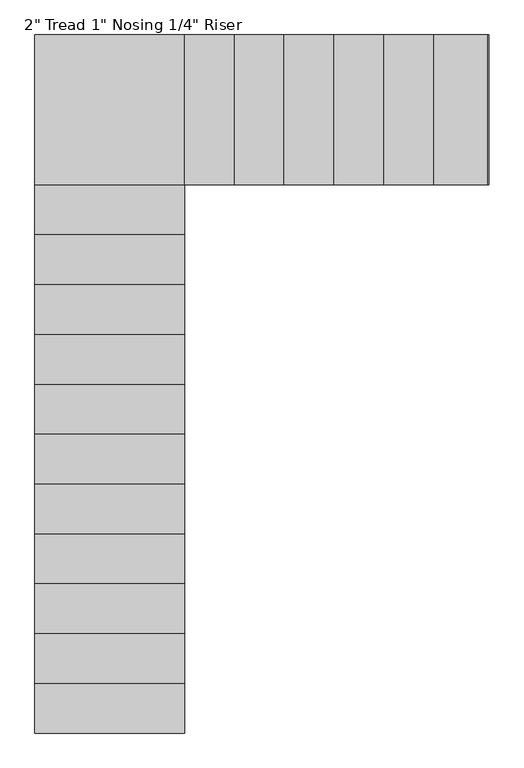
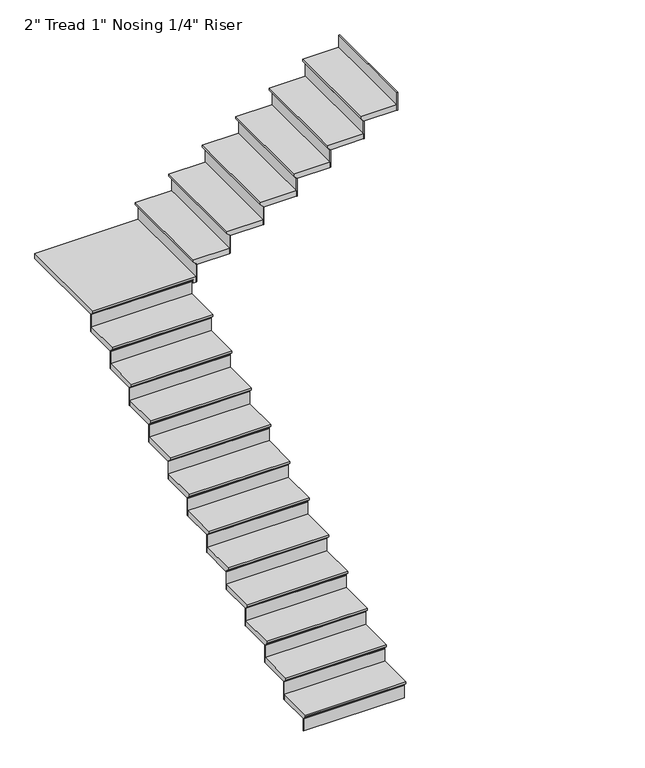
"""IFC4 building model written with IfcOpenShell, lengths in millimetres: stair flight geometry."""

from ifc_helpers import new_model, si_unit, origin, place, context, project, spatial, faceted_brep, source, transform, mapped, element, save


def stair_flight_5b7f780d(model_context):
    return source(origin(), model_context, "Body", "Brep", [
        faceted_brep([(-8401.1607439, -642.5827462, 455.0833333), (-8401.1607439, -642.5827462, 474.1333333), (-9317.1482439, -642.5827462, 474.1333333), (-9317.1482439, -642.5827462, 455.0833333), (-8401.1607439, -617.1827462, 429.6833333), (-9317.1482439, -617.1827462, 429.6833333), (-8401.1607439, -312.3827462, 474.1333333), (-9317.1482439, -312.3827462, 474.1333333), (-9317.1482439, -617.1827462, 423.3333333), (-9317.1482439, -312.3827462, 423.3333333), (-8401.1607439, -312.3827462, 423.3333333), (-8401.1607439, -617.1827462, 423.3333333)], [[[0, 1, 2, 3]], [[4, 0, 3, 5]], [[2, 1, 6, 7]], [[8, 9, 10, 11]], [[2, 7, 9, 8, 5, 3]], [[8, 11, 4, 5]], [[6, 1, 0, 4, 11, 10]], [[7, 6, 10, 9]]]),
        faceted_brep([(-8401.1607439, -617.1827462, 423.3333333), (-8401.1607439, -617.1827462, 304.8), (-8401.1607439, -610.8327462, 304.8), (-8401.1607439, -610.8327462, 423.3333333), (-9317.1482439, -617.1827462, 423.3333333), (-9317.1482439, -610.8327462, 423.3333333), (-9317.1482439, -610.8327462, 304.8), (-9317.1482439, -617.1827462, 304.8)], [[[0, 1, 2, 3]], [[4, 5, 6, 7]], [[1, 0, 4, 7]], [[2, 1, 7, 6]], [[3, 2, 6, 5]], [[0, 3, 5, 4]]]),
        faceted_brep([(-8401.1607439, -312.3827462, 592.6666667), (-8401.1607439, -312.3827462, 423.3333333), (-8401.1607439, -306.0327462, 423.3333333), (-8401.1607439, -306.0327462, 592.6666667), (-9317.1482439, -312.3827462, 592.6666667), (-9317.1482439, -306.0327462, 592.6666667), (-9317.1482439, -306.0327462, 423.3333333), (-9317.1482439, -312.3827462, 423.3333333)], [[[0, 1, 2, 3]], [[4, 5, 6, 7]], [[1, 0, 4, 7]], [[2, 1, 7, 6]], [[3, 2, 6, 5]], [[0, 3, 5, 4]]]),
        faceted_brep([(-9317.1482439, -337.7827462, 643.4666667), (-8401.1607439, -337.7827462, 643.4666667), (-8401.1607439, -7.5827462, 643.4666667), (-9317.1482439, -7.5827462, 643.4666667), (-9317.1482439, -312.3827462, 592.6666667), (-9317.1482439, -7.5827462, 592.6666667), (-8401.1607439, -7.5827462, 592.6666667), (-8401.1607439, -312.3827462, 592.6666667), (-9317.1482439, -312.3827462, 599.0166667), (-9317.1482439, -337.7827462, 624.4166667), (-8401.1607439, -312.3827462, 599.0166667), (-8401.1607439, -337.7827462, 624.4166667)], [[[0, 1, 2, 3]], [[4, 5, 6, 7]], [[0, 3, 5, 4, 8, 9]], [[4, 7, 10, 8]], [[2, 1, 11, 10, 7, 6]], [[3, 2, 6, 5]], [[11, 1, 0, 9]], [[10, 11, 9, 8]]]),
        faceted_brep([(-8401.1607439, -7.5827462, 762.0), (-8401.1607439, -7.5827462, 592.6666667), (-8401.1607439, -1.2327462, 592.6666667), (-8401.1607439, -1.2327462, 762.0), (-9317.1482439, -7.5827462, 762.0), (-9317.1482439, -1.2327462, 762.0), (-9317.1482439, -1.2327462, 592.6666667), (-9317.1482439, -7.5827462, 592.6666667)], [[[0, 1, 2, 3]], [[4, 5, 6, 7]], [[1, 0, 4, 7]], [[2, 1, 7, 6]], [[3, 2, 6, 5]], [[0, 3, 5, 4]]]),
        faceted_brep([(-9317.1482439, -32.9827462, 812.8), (-8401.1607439, -32.9827462, 812.8), (-8401.1607439, 297.2172538, 812.8), (-9317.1482439, 297.2172538, 812.8), (-9317.1482439, -7.5827462, 762.0), (-9317.1482439, 297.2172538, 762.0), (-8401.1607439, 297.2172538, 762.0), (-8401.1607439, -7.5827462, 762.0), (-9317.1482439, -7.5827462, 768.35), (-9317.1482439, -32.9827462, 793.75), (-8401.1607439, -7.5827462, 768.35), (-8401.1607439, -32.9827462, 793.75)], [[[0, 1, 2, 3]], [[4, 5, 6, 7]], [[0, 3, 5, 4, 8, 9]], [[4, 7, 10, 8]], [[2, 1, 11, 10, 7, 6]], [[3, 2, 6, 5]], [[11, 1, 0, 9]], [[10, 11, 9, 8]]]),
        faceted_brep([(-8401.1607439, 297.2172538, 931.3333333), (-8401.1607439, 297.2172538, 762.0), (-8401.1607439, 303.5672538, 762.0), (-8401.1607439, 303.5672538, 931.3333333), (-9317.1482439, 297.2172538, 931.3333333), (-9317.1482439, 303.5672538, 931.3333333), (-9317.1482439, 303.5672538, 762.0), (-9317.1482439, 297.2172538, 762.0)], [[[0, 1, 2, 3]], [[4, 5, 6, 7]], [[1, 0, 4, 7]], [[2, 1, 7, 6]], [[3, 2, 6, 5]], [[0, 3, 5, 4]]]),
        faceted_brep([(-9317.1482439, 271.8172538, 982.1333333), (-8401.1607439, 271.8172538, 982.1333333), (-8401.1607439, 602.0172538, 982.1333333), (-9317.1482439, 602.0172538, 982.1333333), (-9317.1482439, 297.2172538, 931.3333333), (-9317.1482439, 602.0172538, 931.3333333), (-8401.1607439, 602.0172538, 931.3333333), (-8401.1607439, 297.2172538, 931.3333333), (-9317.1482439, 297.2172538, 937.6833333), (-9317.1482439, 271.8172538, 963.0833333), (-8401.1607439, 297.2172538, 937.6833333), (-8401.1607439, 271.8172538, 963.0833333)], [[[0, 1, 2, 3]], [[4, 5, 6, 7]], [[0, 3, 5, 4, 8, 9]], [[4, 7, 10, 8]], [[2, 1, 11, 10, 7, 6]], [[3, 2, 6, 5]], [[11, 1, 0, 9]], [[10, 11, 9, 8]]]),
        faceted_brep([(-8401.1607439, 602.0172538, 1100.6666667), (-8401.1607439, 602.0172538, 931.3333333), (-8401.1607439, 608.3672538, 931.3333333), (-8401.1607439, 608.3672538, 1100.6666667), (-9317.1482439, 602.0172538, 1100.6666667), (-9317.1482439, 608.3672538, 1100.6666667), (-9317.1482439, 608.3672538, 931.3333333), (-9317.1482439, 602.0172538, 931.3333333)], [[[0, 1, 2, 3]], [[4, 5, 6, 7]], [[1, 0, 4, 7]], [[2, 1, 7, 6]], [[3, 2, 6, 5]], [[0, 3, 5, 4]]]),
        faceted_brep([(-9317.1482439, 576.6172538, 1151.4666667), (-8401.1607439, 576.6172538, 1151.4666667), (-8401.1607439, 906.8172538, 1151.4666667), (-9317.1482439, 906.8172538, 1151.4666667), (-9317.1482439, 602.0172538, 1100.6666667), (-9317.1482439, 906.8172538, 1100.6666667), (-8401.1607439, 906.8172538, 1100.6666667), (-8401.1607439, 602.0172538, 1100.6666667), (-9317.1482439, 602.0172538, 1107.0166667), (-9317.1482439, 576.6172538, 1132.4166667), (-8401.1607439, 602.0172538, 1107.0166667), (-8401.1607439, 576.6172538, 1132.4166667)], [[[0, 1, 2, 3]], [[4, 5, 6, 7]], [[0, 3, 5, 4, 8, 9]], [[4, 7, 10, 8]], [[2, 1, 11, 10, 7, 6]], [[3, 2, 6, 5]], [[11, 1, 0, 9]], [[10, 11, 9, 8]]]),
        faceted_brep([(-8401.1607439, 906.8172538, 1270.0), (-8401.1607439, 906.8172538, 1100.6666667), (-8401.1607439, 913.1672538, 1100.6666667), (-8401.1607439, 913.1672538, 1270.0), (-9317.1482439, 906.8172538, 1270.0), (-9317.1482439, 913.1672538, 1270.0), (-9317.1482439, 913.1672538, 1100.6666667), (-9317.1482439, 906.8172538, 1100.6666667)], [[[0, 1, 2, 3]], [[4, 5, 6, 7]], [[1, 0, 4, 7]], [[2, 1, 7, 6]], [[3, 2, 6, 5]], [[0, 3, 5, 4]]]),
        faceted_brep([(-9317.1482439, 881.4172538, 1320.8), (-8401.1607439, 881.4172538, 1320.8), (-8401.1607439, 1211.6172538, 1320.8), (-9317.1482439, 1211.6172538, 1320.8), (-9317.1482439, 906.8172538, 1270.0), (-9317.1482439, 1211.6172538, 1270.0), (-8401.1607439, 1211.6172538, 1270.0), (-8401.1607439, 906.8172538, 1270.0), (-9317.1482439, 906.8172538, 1276.35), (-9317.1482439, 881.4172538, 1301.75), (-8401.1607439, 906.8172538, 1276.35), (-8401.1607439, 881.4172538, 1301.75)], [[[0, 1, 2, 3]], [[4, 5, 6, 7]], [[0, 3, 5, 4, 8, 9]], [[4, 7, 10, 8]], [[2, 1, 11, 10, 7, 6]], [[3, 2, 6, 5]], [[11, 1, 0, 9]], [[10, 11, 9, 8]]]),
        faceted_brep([(-8401.1607439, 1211.6172538, 1439.3333333), (-8401.1607439, 1211.6172538, 1270.0), (-8401.1607439, 1217.9672538, 1270.0), (-8401.1607439, 1217.9672538, 1439.3333333), (-9317.1482439, 1211.6172538, 1439.3333333), (-9317.1482439, 1217.9672538, 1439.3333333), (-9317.1482439, 1217.9672538, 1270.0), (-9317.1482439, 1211.6172538, 1270.0)], [[[0, 1, 2, 3]], [[4, 5, 6, 7]], [[1, 0, 4, 7]], [[2, 1, 7, 6]], [[3, 2, 6, 5]], [[0, 3, 5, 4]]]),
        faceted_brep([(-9317.1482439, 1186.2172538, 1490.1333333), (-8401.1607439, 1186.2172538, 1490.1333333), (-8401.1607439, 1516.4172538, 1490.1333333), (-9317.1482439, 1516.4172538, 1490.1333333), (-9317.1482439, 1211.6172538, 1439.3333333), (-9317.1482439, 1516.4172538, 1439.3333333), (-8401.1607439, 1516.4172538, 1439.3333333), (-8401.1607439, 1211.6172538, 1439.3333333), (-9317.1482439, 1211.6172538, 1445.6833333), (-9317.1482439, 1186.2172538, 1471.0833333), (-8401.1607439, 1211.6172538, 1445.6833333), (-8401.1607439, 1186.2172538, 1471.0833333)], [[[0, 1, 2, 3]], [[4, 5, 6, 7]], [[0, 3, 5, 4, 8, 9]], [[4, 7, 10, 8]], [[2, 1, 11, 10, 7, 6]], [[3, 2, 6, 5]], [[11, 1, 0, 9]], [[10, 11, 9, 8]]]),
        faceted_brep([(-8401.1607439, 1516.4172538, 1608.6666667), (-8401.1607439, 1516.4172538, 1439.3333333), (-8401.1607439, 1522.7672538, 1439.3333333), (-8401.1607439, 1522.7672538, 1608.6666667), (-9317.1482439, 1516.4172538, 1608.6666667), (-9317.1482439, 1522.7672538, 1608.6666667), (-9317.1482439, 1522.7672538, 1439.3333333), (-9317.1482439, 1516.4172538, 1439.3333333)], [[[0, 1, 2, 3]], [[4, 5, 6, 7]], [[1, 0, 4, 7]], [[2, 1, 7, 6]], [[3, 2, 6, 5]], [[0, 3, 5, 4]]]),
        faceted_brep([(-9317.1482439, 1491.0172538, 1659.4666667), (-8401.1607439, 1491.0172538, 1659.4666667), (-8401.1607439, 1821.2172538, 1659.4666667), (-9317.1482439, 1821.2172538, 1659.4666667), (-9317.1482439, 1516.4172538, 1608.6666667), (-9317.1482439, 1821.2172538, 1608.6666667), (-8401.1607439, 1821.2172538, 1608.6666667), (-8401.1607439, 1516.4172538, 1608.6666667), (-9317.1482439, 1516.4172538, 1615.0166667), (-9317.1482439, 1491.0172538, 1640.4166667), (-8401.1607439, 1516.4172538, 1615.0166667), (-8401.1607439, 1491.0172538, 1640.4166667)], [[[0, 1, 2, 3]], [[4, 5, 6, 7]], [[0, 3, 5, 4, 8, 9]], [[4, 7, 10, 8]], [[2, 1, 11, 10, 7, 6]], [[3, 2, 6, 5]], [[11, 1, 0, 9]], [[10, 11, 9, 8]]]),
        faceted_brep([(-8401.1607439, 1821.2172538, 1778.0), (-8401.1607439, 1821.2172538, 1608.6666667), (-8401.1607439, 1827.5672538, 1608.6666667), (-8401.1607439, 1827.5672538, 1778.0), (-9317.1482439, 1821.2172538, 1778.0), (-9317.1482439, 1827.5672538, 1778.0), (-9317.1482439, 1827.5672538, 1608.6666667), (-9317.1482439, 1821.2172538, 1608.6666667)], [[[0, 1, 2, 3]], [[4, 5, 6, 7]], [[1, 0, 4, 7]], [[2, 1, 7, 6]], [[3, 2, 6, 5]], [[0, 3, 5, 4]]]),
        faceted_brep([(-9317.1482439, 1795.8172538, 1828.8), (-8401.1607439, 1795.8172538, 1828.8), (-8401.1607439, 2126.0172538, 1828.8), (-9317.1482439, 2126.0172538, 1828.8), (-9317.1482439, 1821.2172538, 1778.0), (-9317.1482439, 2126.0172538, 1778.0), (-8401.1607439, 2126.0172538, 1778.0), (-8401.1607439, 1821.2172538, 1778.0), (-9317.1482439, 1821.2172538, 1784.35), (-9317.1482439, 1795.8172538, 1809.75), (-8401.1607439, 1821.2172538, 1784.35), (-8401.1607439, 1795.8172538, 1809.75)], [[[0, 1, 2, 3]], [[4, 5, 6, 7]], [[0, 3, 5, 4, 8, 9]], [[4, 7, 10, 8]], [[2, 1, 11, 10, 7, 6]], [[3, 2, 6, 5]], [[11, 1, 0, 9]], [[10, 11, 9, 8]]]),
        faceted_brep([(-8401.1607439, 2126.0172538, 1947.3333333), (-8401.1607439, 2126.0172538, 1778.0), (-8401.1607439, 2132.3672538, 1778.0), (-8401.1607439, 2132.3672538, 1947.3333333), (-9317.1482439, 2126.0172538, 1947.3333333), (-9317.1482439, 2132.3672538, 1947.3333333), (-9317.1482439, 2132.3672538, 1778.0), (-9317.1482439, 2126.0172538, 1778.0)], [[[0, 1, 2, 3]], [[4, 5, 6, 7]], [[1, 0, 4, 7]], [[2, 1, 7, 6]], [[3, 2, 6, 5]], [[0, 3, 5, 4]]]),
        faceted_brep([(-9317.1482439, 2100.6172538, 1998.1333333), (-8401.1607439, 2100.6172538, 1998.1333333), (-8401.1607439, 2430.8172538, 1998.1333333), (-9317.1482439, 2430.8172538, 1998.1333333), (-9317.1482439, 2126.0172538, 1947.3333333), (-9317.1482439, 2430.8172538, 1947.3333333), (-8401.1607439, 2430.8172538, 1947.3333333), (-8401.1607439, 2126.0172538, 1947.3333333), (-9317.1482439, 2126.0172538, 1953.6833333), (-9317.1482439, 2100.6172538, 1979.0833333), (-8401.1607439, 2126.0172538, 1953.6833333), (-8401.1607439, 2100.6172538, 1979.0833333)], [[[0, 1, 2, 3]], [[4, 5, 6, 7]], [[0, 3, 5, 4, 8, 9]], [[4, 7, 10, 8]], [[2, 1, 11, 10, 7, 6]], [[3, 2, 6, 5]], [[11, 1, 0, 9]], [[10, 11, 9, 8]]]),
        faceted_brep([(-8401.1607439, 2430.8172538, 2116.6666667), (-8401.1607439, 2430.8172538, 1947.3333333), (-8401.1607439, 2437.1672538, 1947.3333333), (-8401.1607439, 2437.1672538, 2116.6666667), (-9317.1482439, 2430.8172538, 2116.6666667), (-9317.1482439, 2437.1672538, 2116.6666667), (-9317.1482439, 2437.1672538, 1947.3333333), (-9317.1482439, 2430.8172538, 1947.3333333)], [[[0, 1, 2, 3]], [[4, 5, 6, 7]], [[1, 0, 4, 7]], [[2, 1, 7, 6]], [[3, 2, 6, 5]], [[0, 3, 5, 4]]]),
        faceted_brep([(-9317.1482439, 2405.4172538, 2167.4666667), (-8401.1607439, 2405.4172538, 2167.4666667), (-8401.1607439, 2735.6172538, 2167.4666667), (-9317.1482439, 2735.6172538, 2167.4666667), (-9317.1482439, 2430.8172538, 2116.6666667), (-9317.1482439, 2735.6172538, 2116.6666667), (-8401.1607439, 2735.6172538, 2116.6666667), (-8401.1607439, 2430.8172538, 2116.6666667), (-9317.1482439, 2430.8172538, 2123.0166667), (-9317.1482439, 2405.4172538, 2148.4166667), (-8401.1607439, 2430.8172538, 2123.0166667), (-8401.1607439, 2405.4172538, 2148.4166667)], [[[0, 1, 2, 3]], [[4, 5, 6, 7]], [[0, 3, 5, 4, 8, 9]], [[4, 7, 10, 8]], [[2, 1, 11, 10, 7, 6]], [[3, 2, 6, 5]], [[11, 1, 0, 9]], [[10, 11, 9, 8]]]),
        faceted_brep([(-8401.1607439, 2735.6172538, 2286.0), (-8401.1607439, 2735.6172538, 2116.6666667), (-8401.1607439, 2741.9672538, 2116.6666667), (-8401.1607439, 2741.9672538, 2286.0), (-9317.1482439, 2735.6172538, 2286.0), (-9317.1482439, 2741.9672538, 2286.0), (-9317.1482439, 2741.9672538, 2116.6666667), (-9317.1482439, 2735.6172538, 2116.6666667)], [[[0, 1, 2, 3]], [[4, 5, 6, 7]], [[1, 0, 4, 7]], [[2, 1, 7, 6]], [[3, 2, 6, 5]], [[0, 3, 5, 4]]]),
        faceted_brep([(-8375.7607439, 3624.6172538, 2336.8), (-9317.1482439, 3624.6172538, 2336.8), (-9317.1482439, 2710.2172538, 2336.8), (-8375.7607439, 2710.2172538, 2336.8), (-9317.1482439, 3624.6172538, 2286.0), (-8375.7607439, 3624.6172538, 2286.0), (-8375.7607439, 2710.2172538, 2286.0), (-8401.1607439, 2710.2172538, 2286.0), (-8401.1607439, 2735.6172538, 2286.0), (-9317.1482439, 2735.6172538, 2286.0), (-9317.1482439, 2735.6172538, 2292.35), (-9317.1482439, 2710.2172538, 2317.75), (-8401.1607439, 2735.6172538, 2292.35), (-8401.1607439, 2710.2172538, 2317.75)], [[[0, 1, 2, 3]], [[4, 5, 6, 7, 8, 9]], [[1, 0, 5, 4]], [[2, 1, 4, 9, 10, 11]], [[9, 8, 12, 10]], [[8, 7, 13, 12]], [[3, 2, 11, 13, 7, 6]], [[0, 3, 6, 5]], [[11, 10, 12, 13]]]),
        faceted_brep([(-8375.7607439, 2710.2172538, 2455.3333333), (-8375.7607439, 2710.2172538, 2286.0), (-8369.4107439, 2710.2172538, 2286.0), (-8369.4107439, 2710.2172538, 2455.3333333), (-8375.7607439, 3624.6172538, 2455.3333333), (-8369.4107439, 3624.6172538, 2455.3333333), (-8369.4107439, 3624.6172538, 2286.0), (-8375.7607439, 3624.6172538, 2286.0)], [[[0, 1, 2, 3]], [[4, 5, 6, 7]], [[1, 0, 4, 7]], [[2, 1, 7, 6]], [[3, 2, 6, 5]], [[0, 3, 5, 4]]]),
        faceted_brep([(-8401.1607439, 3624.6172538, 2506.1333333), (-8401.1607439, 2710.2172538, 2506.1333333), (-8070.9607439, 2710.2172538, 2506.1333333), (-8070.9607439, 3624.6172538, 2506.1333333), (-8375.7607439, 3624.6172538, 2455.3333333), (-8070.9607439, 3624.6172538, 2455.3333333), (-8070.9607439, 2710.2172538, 2455.3333333), (-8375.7607439, 2710.2172538, 2455.3333333), (-8375.7607439, 3624.6172538, 2461.6833333), (-8401.1607439, 3624.6172538, 2487.0833333), (-8375.7607439, 2710.2172538, 2461.6833333), (-8401.1607439, 2710.2172538, 2487.0833333)], [[[0, 1, 2, 3]], [[4, 5, 6, 7]], [[0, 3, 5, 4, 8, 9]], [[4, 7, 10, 8]], [[2, 1, 11, 10, 7, 6]], [[3, 2, 6, 5]], [[11, 1, 0, 9]], [[10, 11, 9, 8]]]),
        faceted_brep([(-8070.9607439, 2710.2172538, 2624.6666667), (-8070.9607439, 2710.2172538, 2455.3333333), (-8064.6107439, 2710.2172538, 2455.3333333), (-8064.6107439, 2710.2172538, 2624.6666667), (-8070.9607439, 3624.6172538, 2624.6666667), (-8064.6107439, 3624.6172538, 2624.6666667), (-8064.6107439, 3624.6172538, 2455.3333333), (-8070.9607439, 3624.6172538, 2455.3333333)], [[[0, 1, 2, 3]], [[4, 5, 6, 7]], [[1, 0, 4, 7]], [[2, 1, 7, 6]], [[3, 2, 6, 5]], [[0, 3, 5, 4]]]),
        faceted_brep([(-8096.3607439, 3624.6172538, 2675.4666667), (-8096.3607439, 2710.2172538, 2675.4666667), (-7766.1607439, 2710.2172538, 2675.4666667), (-7766.1607439, 3624.6172538, 2675.4666667), (-8070.9607439, 3624.6172538, 2624.6666667), (-7766.1607439, 3624.6172538, 2624.6666667), (-7766.1607439, 2710.2172538, 2624.6666667), (-8070.9607439, 2710.2172538, 2624.6666667), (-8070.9607439, 3624.6172538, 2631.0166667), (-8096.3607439, 3624.6172538, 2656.4166667), (-8070.9607439, 2710.2172538, 2631.0166667), (-8096.3607439, 2710.2172538, 2656.4166667)], [[[0, 1, 2, 3]], [[4, 5, 6, 7]], [[0, 3, 5, 4, 8, 9]], [[4, 7, 10, 8]], [[2, 1, 11, 10, 7, 6]], [[3, 2, 6, 5]], [[11, 1, 0, 9]], [[10, 11, 9, 8]]]),
        faceted_brep([(-7766.1607439, 2710.2172538, 2794.0), (-7766.1607439, 2710.2172538, 2624.6666667), (-7759.8107439, 2710.2172538, 2624.6666667), (-7759.8107439, 2710.2172538, 2794.0), (-7766.1607439, 3624.6172538, 2794.0), (-7759.8107439, 3624.6172538, 2794.0), (-7759.8107439, 3624.6172538, 2624.6666667), (-7766.1607439, 3624.6172538, 2624.6666667)], [[[0, 1, 2, 3]], [[4, 5, 6, 7]], [[1, 0, 4, 7]], [[2, 1, 7, 6]], [[3, 2, 6, 5]], [[0, 3, 5, 4]]]),
        faceted_brep([(-7791.5607439, 3624.6172538, 2844.8), (-7791.5607439, 2710.2172538, 2844.8), (-7461.3607439, 2710.2172538, 2844.8), (-7461.3607439, 3624.6172538, 2844.8), (-7766.1607439, 3624.6172538, 2794.0), (-7461.3607439, 3624.6172538, 2794.0), (-7461.3607439, 2710.2172538, 2794.0), (-7766.1607439, 2710.2172538, 2794.0), (-7766.1607439, 3624.6172538, 2800.35), (-7791.5607439, 3624.6172538, 2825.75), (-7766.1607439, 2710.2172538, 2800.35), (-7791.5607439, 2710.2172538, 2825.75)], [[[0, 1, 2, 3]], [[4, 5, 6, 7]], [[0, 3, 5, 4, 8, 9]], [[4, 7, 10, 8]], [[2, 1, 11, 10, 7, 6]], [[3, 2, 6, 5]], [[11, 1, 0, 9]], [[10, 11, 9, 8]]]),
        faceted_brep([(-7461.3607439, 2710.2172538, 2963.3333333), (-7461.3607439, 2710.2172538, 2794.0), (-7455.0107439, 2710.2172538, 2794.0), (-7455.0107439, 2710.2172538, 2963.3333333), (-7461.3607439, 3624.6172538, 2963.3333333), (-7455.0107439, 3624.6172538, 2963.3333333), (-7455.0107439, 3624.6172538, 2794.0), (-7461.3607439, 3624.6172538, 2794.0)], [[[0, 1, 2, 3]], [[4, 5, 6, 7]], [[1, 0, 4, 7]], [[2, 1, 7, 6]], [[3, 2, 6, 5]], [[0, 3, 5, 4]]]),
        faceted_brep([(-7486.7607439, 3624.6172538, 3014.1333333), (-7486.7607439, 2710.2172538, 3014.1333333), (-7156.5607439, 2710.2172538, 3014.1333333), (-7156.5607439, 3624.6172538, 3014.1333333), (-7461.3607439, 3624.6172538, 2963.3333333), (-7156.5607439, 3624.6172538, 2963.3333333), (-7156.5607439, 2710.2172538, 2963.3333333), (-7461.3607439, 2710.2172538, 2963.3333333), (-7461.3607439, 3624.6172538, 2969.6833333), (-7486.7607439, 3624.6172538, 2995.0833333), (-7461.3607439, 2710.2172538, 2969.6833333), (-7486.7607439, 2710.2172538, 2995.0833333)], [[[0, 1, 2, 3]], [[4, 5, 6, 7]], [[0, 3, 5, 4, 8, 9]], [[4, 7, 10, 8]], [[2, 1, 11, 10, 7, 6]], [[3, 2, 6, 5]], [[11, 1, 0, 9]], [[10, 11, 9, 8]]]),
        faceted_brep([(-7156.5607439, 2710.2172538, 3132.6666667), (-7156.5607439, 2710.2172538, 2963.3333333), (-7150.2107439, 2710.2172538, 2963.3333333), (-7150.2107439, 2710.2172538, 3132.6666667), (-7156.5607439, 3624.6172538, 3132.6666667), (-7150.2107439, 3624.6172538, 3132.6666667), (-7150.2107439, 3624.6172538, 2963.3333333), (-7156.5607439, 3624.6172538, 2963.3333333)], [[[0, 1, 2, 3]], [[4, 5, 6, 7]], [[1, 0, 4, 7]], [[2, 1, 7, 6]], [[3, 2, 6, 5]], [[0, 3, 5, 4]]]),
        faceted_brep([(-7181.9607439, 3624.6172538, 3183.4666667), (-7181.9607439, 2710.2172538, 3183.4666667), (-6851.7607439, 2710.2172538, 3183.4666667), (-6851.7607439, 3624.6172538, 3183.4666667), (-7156.5607439, 3624.6172538, 3132.6666667), (-6851.7607439, 3624.6172538, 3132.6666667), (-6851.7607439, 2710.2172538, 3132.6666667), (-7156.5607439, 2710.2172538, 3132.6666667), (-7156.5607439, 3624.6172538, 3139.0166667), (-7181.9607439, 3624.6172538, 3164.4166667), (-7156.5607439, 2710.2172538, 3139.0166667), (-7181.9607439, 2710.2172538, 3164.4166667)], [[[0, 1, 2, 3]], [[4, 5, 6, 7]], [[0, 3, 5, 4, 8, 9]], [[4, 7, 10, 8]], [[2, 1, 11, 10, 7, 6]], [[3, 2, 6, 5]], [[11, 1, 0, 9]], [[10, 11, 9, 8]]]),
        faceted_brep([(-6851.7607439, 2710.2172538, 3302.0), (-6851.7607439, 2710.2172538, 3132.6666667), (-6845.4107439, 2710.2172538, 3132.6666667), (-6845.4107439, 2710.2172538, 3302.0), (-6851.7607439, 3624.6172538, 3302.0), (-6845.4107439, 3624.6172538, 3302.0), (-6845.4107439, 3624.6172538, 3132.6666667), (-6851.7607439, 3624.6172538, 3132.6666667)], [[[0, 1, 2, 3]], [[4, 5, 6, 7]], [[1, 0, 4, 7]], [[2, 1, 7, 6]], [[3, 2, 6, 5]], [[0, 3, 5, 4]]]),
        faceted_brep([(-6546.9607439, 2710.2172538, 3471.3333333), (-6546.9607439, 2710.2172538, 3302.0), (-6540.6107439, 2710.2172538, 3302.0), (-6540.6107439, 2710.2172538, 3471.3333333), (-6546.9607439, 3624.6172538, 3471.3333333), (-6540.6107439, 3624.6172538, 3471.3333333), (-6540.6107439, 3624.6172538, 3302.0), (-6546.9607439, 3624.6172538, 3302.0)], [[[0, 1, 2, 3]], [[4, 5, 6, 7]], [[1, 0, 4, 7]], [[2, 1, 7, 6]], [[3, 2, 6, 5]], [[0, 3, 5, 4]]]),
        faceted_brep([(-6877.1607439, 3624.6172538, 3352.8), (-6877.1607439, 2710.2172538, 3352.8), (-6546.9607439, 2710.2172538, 3352.8), (-6546.9607439, 3624.6172538, 3352.8), (-6851.7607439, 3624.6172538, 3302.0), (-6546.9607439, 3624.6172538, 3302.0), (-6546.9607439, 2710.2172538, 3302.0), (-6851.7607439, 2710.2172538, 3302.0), (-6851.7607439, 3624.6172538, 3308.35), (-6877.1607439, 3624.6172538, 3333.75), (-6851.7607439, 2710.2172538, 3308.35), (-6877.1607439, 2710.2172538, 3333.75)], [[[0, 1, 2, 3]], [[4, 5, 6, 7]], [[0, 3, 5, 4, 8, 9]], [[4, 7, 10, 8]], [[2, 1, 11, 10, 7, 6]], [[3, 2, 6, 5]], [[11, 1, 0, 9]], [[10, 11, 9, 8]]]),
    ])


if __name__ == "__main__":
    model = new_model("IFC4")
    model_context = context("Model", 3, world=origin())
    ifc_project = project(units=[si_unit("LENGTHUNIT", "METRE", prefix="MILLI")], contexts=[model_context])
    site = spatial("IfcSite", under=ifc_project)
    building = spatial("IfcBuilding", under=site)
    placement = place(None, origin())
    stair_flight_shape = stair_flight_5b7f780d(model_context)
    element("IfcStairFlight", 1, ObjectType="2\" Tread 1\" Nosing 1/4\" Riser", at=placement, inside=building, context=model_context, shape_type="MappedRepresentation", body=[
        mapped(stair_flight_shape, transform((0.0, 0.0, 0.0), x_axis=(1.0, 0.0, 0.0), y_axis=(0.0, 1.0, 0.0), z_axis=(0.0, 0.0, 1.0))),
    ])
    save(model, "model.ifc")

# Revit data of these elements
# Element 1 (IfcStairFlight, "2\" Tread 1\" Nosing 1/4\" Riser")
#   Materials on its faces: "MARBLE PAINT"
# Materials
#   "MARBLE PAINT": class "Generic", colour RGB 120 120 120, transparency 0, Cost = 0
